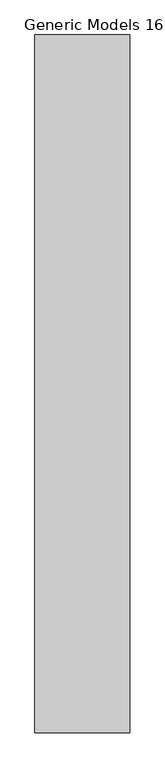
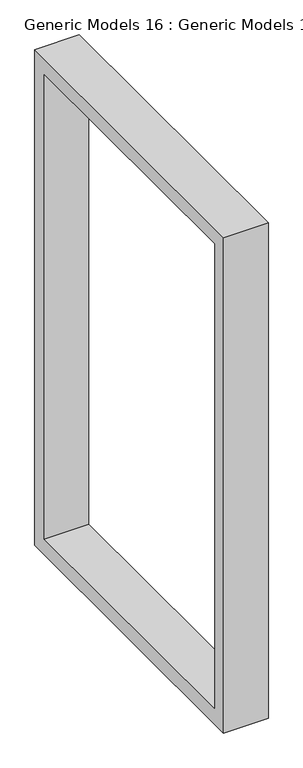
"""IFC4 building model written with IfcOpenShell, lengths in millimetres: proxy geometry, Generic Models 16 : Generic Models 16."""

from ifc_helpers import new_model, si_unit, frame, origin, place, context, project, spatial, polyline, outline, extrude, source, transform, mapped, element, save


def generic_models_16_generic_models_16_15e574d3(model_context):
    return source(origin(), model_context, "Body", "SweptSolid", [
        extrude(outline(polyline([(8991.6641252, 304.8), (8991.6641252, 5181.6), (12039.6641252, 5181.6), (12039.6641252, 304.8), (8991.6641252, 304.8)]), holes=[polyline([(9144.0641252, 5029.2), (9144.0641252, 457.2), (11887.2641252, 457.2), (11887.2641252, 5029.2), (9144.0641252, 5029.2)])]), frame((-2245.1874287, 0.0, 0.0), z_axis=(1.0, 0.0, 0.0), x_axis=(0.0, 1.0, 0.0)), (0.0, 0.0, 1.0), 414.9593979),
    ])


if __name__ == "__main__":
    model = new_model("IFC4")
    model_context = context("Model", 3, world=origin())
    ifc_project = project(units=[si_unit("LENGTHUNIT", "METRE", prefix="MILLI")], contexts=[model_context])
    site = spatial("IfcSite", under=ifc_project)
    building = spatial("IfcBuilding", under=site)
    placement = place(None, origin())
    generic_models_16_generic_models_16_shape = generic_models_16_generic_models_16_15e574d3(model_context)
    element("IfcBuildingElementProxy", 1, Name="Generic Models 16 : Generic Models 16", ObjectType="Generic Models 16 : Generic Models 16", at=placement, inside=building, context=model_context, shape_type="MappedRepresentation", body=[
        mapped(generic_models_16_generic_models_16_shape, transform((0.0, 0.0, 0.0), x_axis=(1.0, 0.0, 0.0), y_axis=(0.0, 1.0, 0.0), z_axis=(0.0, 0.0, 1.0))),
    ])
    save(model, "model.ifc")

# Revit data of these elements
# Element 1 (IfcBuildingElementProxy, "Generic Models 16 : Generic Models 16")
#   Materials on its faces: "chocolate brown"
# Materials
#   "chocolate brown": class "Generic", colour RGB 120 120 120, transparency 0, Cost = 0
